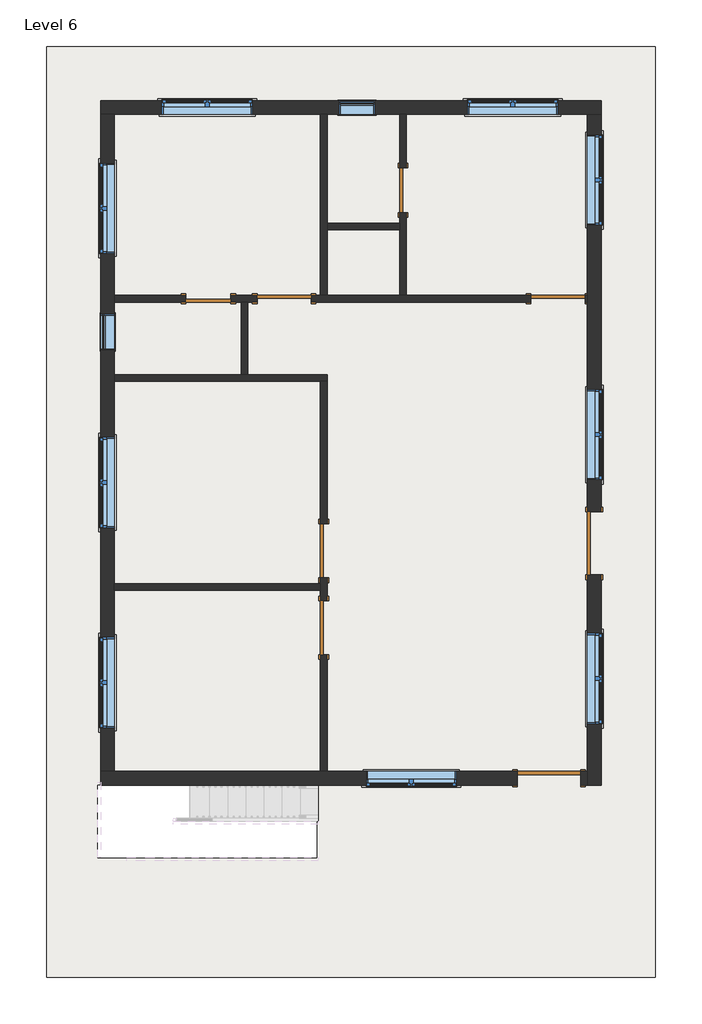
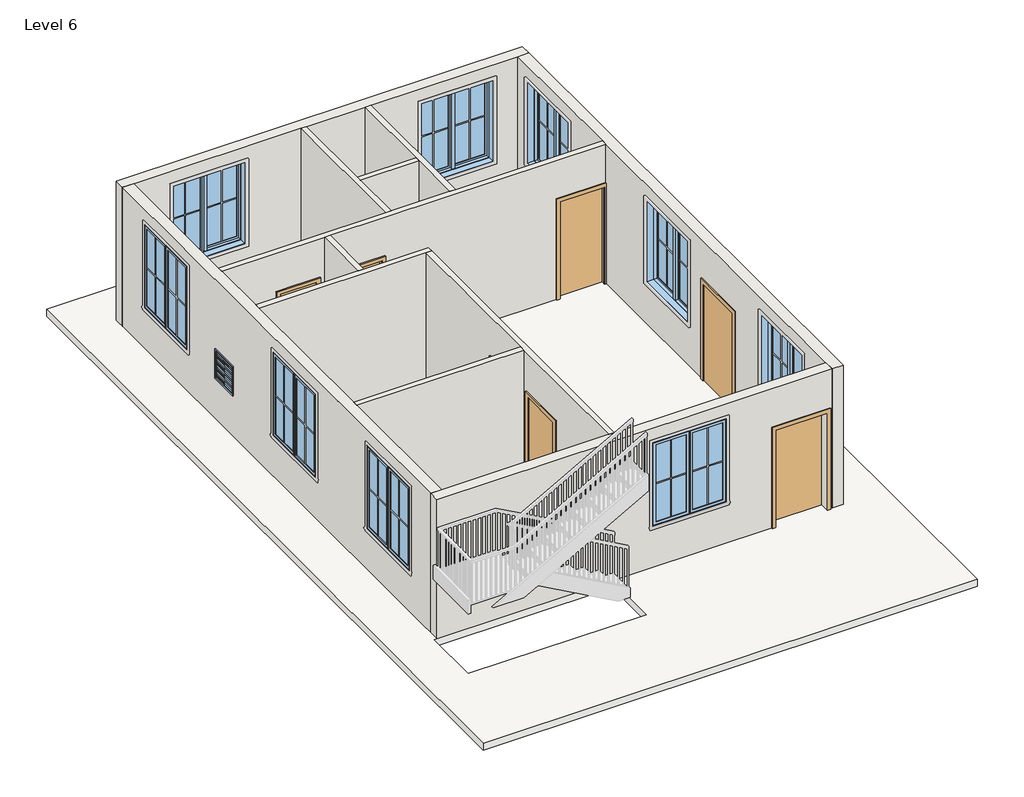
# One storey, part 1 of 3: 12 walls, 11 windows, 8 doors, 1 roof.
"""IFC4 building model written with IfcOpenShell, lengths in millimetres."""

from ifc_helpers import new_model, si_unit, frame, origin, place, context, project, spatial, polyline, outline, extrude, faceted_brep, transform, mapped, element, save
from components import door_78caadf7, single_flush_door_3_e5f9f3c4, single_flush_door_3_305aa2a5, door_9d399b00, door_0848dd25, window_casement_double_win_5_f93960c7, window_f2d8fef0

model = new_model("IFC4")

# Units and contexts
model_context = context("Model", 3, world=origin())
ifc_project = project(units=[si_unit("LENGTHUNIT", "METRE", prefix="MILLI")], contexts=[model_context])

# Site, building, storey
site = spatial("IfcSite", under=ifc_project)
building = spatial("IfcBuilding", under=site)
storey = spatial("IfcBuildingStorey", under=building, Name="Level 6", Elevation=12801.6)

# Doors
placement = place(None, origin())
door_shape = door_78caadf7(model_context)
element("IfcDoor", 1, ObjectType="Single-Flush : DOOR 2'6\"", at=placement, inside=storey, context=model_context, shape_type="MappedRepresentation", body=[
    mapped(door_shape, transform((-377.1698569, 4707.5566963, 12801.6), x_axis=(0.0, -1.0, 0.0), y_axis=(1.0, 0.0, 0.0), z_axis=(0.0, 0.0, 1.0))),
])
element("IfcDoor", 2, ObjectType="Single-Flush : DOOR 2'6\"", at=placement, inside=storey, context=model_context, shape_type="MappedRepresentation", body=[
    mapped(door_shape, transform((-3653.7698569, 2878.7566963, 12801.6), x_axis=(1.0, 0.0, 0.0), y_axis=(0.0, 1.0, 0.0), z_axis=(0.0, 0.0, 1.0))),
])
single_flush_door_3_shape = single_flush_door_3_e5f9f3c4(model_context)
element("IfcDoor", 3, ObjectType="Single-Flush : DOOR 3'", at=placement, inside=storey, context=model_context, shape_type="MappedRepresentation", body=[
    mapped(single_flush_door_3_shape, transform((-2377.4198569, 2878.7566963, 12801.6), x_axis=(1.0, 0.0, 0.0), y_axis=(0.0, 1.0, 0.0), z_axis=(0.0, 0.0, 1.0))),
])
element("IfcDoor", 4, ObjectType="Single-Flush : DOOR 3'", at=placement, inside=storey, context=model_context, shape_type="MappedRepresentation", body=[
    mapped(single_flush_door_3_shape, transform((2232.6801431, 2878.7566963, 12801.6), x_axis=(1.0, 0.0, 0.0), y_axis=(0.0, 1.0, 0.0), z_axis=(0.0, 0.0, 1.0))),
])
element("IfcDoor", 5, ObjectType="Single-Flush : DOOR 3'", at=placement, inside=storey, context=model_context, shape_type="MappedRepresentation", body=[
    mapped(single_flush_door_3_shape, transform((-1710.6698569, -2658.4433037, 12801.6), x_axis=(0.0, 1.0, 0.0), y_axis=(-1.0, 0.0, 0.0), z_axis=(0.0, 0.0, 1.0))),
])
single_flush_door_3_2_shape = single_flush_door_3_305aa2a5(model_context)
element("IfcDoor", 6, ObjectType="Single-Flush : DOOR 3'", at=placement, inside=storey, context=model_context, shape_type="MappedRepresentation", body=[
    mapped(single_flush_door_3_2_shape, transform((-1710.6698569, -1363.0433037, 12801.6), x_axis=(0.0, -1.0, 0.0), y_axis=(1.0, 0.0, 0.0), z_axis=(0.0, 0.0, 1.0))),
])
door_2_shape = door_9d399b00(model_context)
element("IfcDoor", 7, ObjectType="Single-Flush : DOOR 3'6\"", at=placement, inside=storey, context=model_context, shape_type="MappedRepresentation", body=[
    mapped(door_2_shape, transform((2080.2801431, -5192.0933037, 12801.6), x_axis=(1.0, 0.0, 0.0), y_axis=(0.0, 1.0, 0.0), z_axis=(0.0, 0.0, 1.0))),
])
door_3_shape = door_0848dd25(model_context)
element("IfcDoor", 8, ObjectType="Single-Flush : DOOR 3'6\"", at=placement, inside=storey, context=model_context, shape_type="MappedRepresentation", body=[
    mapped(door_3_shape, transform((2842.2801431, -1236.0433037, 12801.6), x_axis=(0.0, -1.0, 0.0), y_axis=(1.0, 0.0, 0.0), z_axis=(0.0, 0.0, 1.0))),
])

# Roof
element("IfcRoof", 9, ObjectType="ROOF 6\"", at=placement, inside=storey, context=model_context, shape_type="SweptSolid", body=[
    extrude(outline(polyline([(-6377.9198569, -8544.8933037), (-6377.9198569, 7126.9066963), (3870.9801431, 7126.9066963), (3870.9801431, -8544.8933037), (-6377.9198569, -8544.8933037)]), holes=[polyline([(-5514.3198569, -5306.3933037), (-5514.3198569, -6525.5933037), (-1831.3198569, -6525.5933037), (-1831.3198569, -5306.3933037), (-5514.3198569, -5306.3933037)])]), frame((0.0, 0.0, 12649.2), z_axis=(0.0, 0.0, 1.0), x_axis=(1.0, 0.0, 0.0)), (0.0, 0.0, 1.0), 152.4),
])

# Walls
element("IfcWall", 10, ObjectType="WALL 4.5\"", at=placement, inside=storey, context=model_context, shape_type="Brep", body=[
    faceted_brep([(2689.8801431, 2821.6066963, 14935.2), (2689.8801431, 2821.6066963, 12801.6), (2727.9801431, 2821.6066963, 12801.6), (2727.9801431, 2821.6066963, 15849.6), (-2987.0198569, 2821.6066963, 15849.6), (-3101.3198569, 2821.6066963, 15849.6), (-5234.9198569, 2821.6066963, 15849.6), (-5234.9198569, 2821.6066963, 12801.6), (-4034.7698569, 2821.6066963, 12801.6), (-4034.7698569, 2821.6066963, 14935.2), (-3272.7698569, 2821.6066963, 14935.2), (-3272.7698569, 2821.6066963, 12801.6), (-3101.3198569, 2821.6066963, 12801.6), (-2987.0198569, 2821.6066963, 12801.6), (-2834.6198569, 2821.6066963, 12801.6), (-2834.6198569, 2821.6066963, 14935.2), (-1920.2198569, 2821.6066963, 14935.2), (-1920.2198569, 2821.6066963, 12801.6), (1775.4801431, 2821.6066963, 12801.6), (1775.4801431, 2821.6066963, 14935.2), (2727.9801431, 2935.9066963, 12801.6), (2689.8801431, 2935.9066963, 12801.6), (2689.8801431, 2935.9066963, 14935.2), (1775.4801431, 2935.9066963, 14935.2), (1775.4801431, 2935.9066963, 12801.6), (-320.0198569, 2935.9066963, 12801.6), (-434.3198569, 2935.9066963, 12801.6), (-1653.5198569, 2935.9066963, 12801.6), (-1767.8198569, 2935.9066963, 12801.6), (-1920.2198569, 2935.9066963, 12801.6), (-1920.2198569, 2935.9066963, 14935.2), (-2834.6198569, 2935.9066963, 14935.2), (-2834.6198569, 2935.9066963, 12801.6), (-3272.7698569, 2935.9066963, 12801.6), (-3272.7698569, 2935.9066963, 14935.2), (-4034.7698569, 2935.9066963, 14935.2), (-4034.7698569, 2935.9066963, 12801.6), (-5234.9198569, 2935.9066963, 12801.6), (-5234.9198569, 2935.9066963, 15849.6), (-1767.8198569, 2935.9066963, 15849.6), (-1653.5198569, 2935.9066963, 15849.6), (-434.3198569, 2935.9066963, 15849.6), (-320.0198569, 2935.9066963, 15849.6), (2727.9801431, 2935.9066963, 15849.6)], [[[0, 1, 2, 3, 4, 5, 6, 7, 8, 9, 10, 11, 12, 13, 14, 15, 16, 17, 18, 19]], [[20, 21, 22, 23, 24, 25, 26, 27, 28, 29, 30, 31, 32, 33, 34, 35, 36, 37, 38, 39, 40, 41, 42, 43]], [[8, 7, 37, 36]], [[14, 13, 12, 11, 33, 32]], [[18, 17, 29, 28, 27, 26, 25, 24]], [[2, 1, 21, 20]], [[3, 2, 20, 43]], [[7, 6, 38, 37]], [[34, 33, 11, 10]], [[35, 34, 10, 9]], [[36, 35, 9, 8]], [[30, 29, 17, 16]], [[31, 30, 16, 15]], [[32, 31, 15, 14]], [[22, 21, 1, 0]], [[23, 22, 0, 19]], [[24, 23, 19, 18]], [[6, 5, 4, 3, 43, 42, 41, 40, 39, 38]]]),
])
element("IfcWall", 11, ObjectType="WALL 4.5\"", at=placement, inside=storey, context=model_context, shape_type="Brep", body=[
    faceted_brep([(-1767.8198569, 5983.9066963, 12801.6), (-1767.8198569, 2935.9066963, 12801.6), (-1767.8198569, 2935.9066963, 15849.6), (-1767.8198569, 5983.9066963, 15849.6), (-1653.5198569, 5983.9066963, 12801.6), (-1653.5198569, 5983.9066963, 15849.6), (-1653.5198569, 4155.1066963, 15849.6), (-1653.5198569, 4040.8066963, 15849.6), (-1653.5198569, 2935.9066963, 15849.6), (-1653.5198569, 2935.9066963, 12801.6), (-1653.5198569, 4040.8066963, 12801.6), (-1653.5198569, 4155.1066963, 12801.6)], [[[0, 1, 2, 3]], [[4, 5, 6, 7, 8, 9, 10, 11]], [[1, 0, 4, 11, 10, 9]], [[0, 3, 5, 4]], [[2, 1, 9, 8]], [[3, 2, 8, 7, 6, 5]]]),
])
element("IfcWall", 12, ObjectType="WALL 4.5\"", at=placement, inside=storey, context=model_context, shape_type="Brep", body=[
    faceted_brep([(-320.0198569, 2935.9066963, 12801.6), (-320.0198569, 4326.5566963, 12801.6), (-320.0198569, 4326.5566963, 14935.2), (-320.0198569, 5088.5566963, 14935.2), (-320.0198569, 5088.5566963, 12801.6), (-320.0198569, 5983.9066963, 12801.6), (-320.0198569, 5983.9066963, 15849.6), (-320.0198569, 2935.9066963, 15849.6), (-434.3198569, 4326.5566963, 14935.2), (-434.3198569, 4326.5566963, 12801.6), (-434.3198569, 4155.1066963, 12801.6), (-434.3198569, 4040.8066963, 12801.6), (-434.3198569, 2935.9066963, 12801.6), (-434.3198569, 2935.9066963, 15849.6), (-434.3198569, 4040.8066963, 15849.6), (-434.3198569, 4155.1066963, 15849.6), (-434.3198569, 5983.9066963, 15849.6), (-434.3198569, 5983.9066963, 12801.6), (-434.3198569, 5088.5566963, 12801.6), (-434.3198569, 5088.5566963, 14935.2)], [[[0, 1, 2, 3, 4, 5, 6, 7]], [[8, 9, 10, 11, 12, 13, 14, 15, 16, 17, 18, 19]], [[18, 17, 5, 4]], [[12, 11, 10, 9, 1, 0]], [[6, 5, 17, 16]], [[0, 7, 13, 12]], [[2, 1, 9, 8]], [[3, 2, 8, 19]], [[4, 3, 19, 18]], [[7, 6, 16, 15, 14, 13]]]),
])
element("IfcWall", 13, ObjectType="WALL 4.5\"", at=placement, inside=storey, context=model_context, shape_type="SweptSolid", body=[
    extrude(outline(polyline([(-434.3198569, 4040.8066963), (-1653.5198569, 4040.8066963), (-1653.5198569, 4155.1066963), (-434.3198569, 4155.1066963), (-434.3198569, 4040.8066963)])), frame((0.0, 0.0, 12801.6), z_axis=(0.0, 0.0, 1.0), x_axis=(1.0, 0.0, 0.0)), (0.0, 0.0, 1.0), 3048.0),
])
element("IfcWall", 14, ObjectType="WALL 4.5\"", at=placement, inside=storey, context=model_context, shape_type="Brep", body=[
    faceted_brep([(-5234.9198569, 1488.1066963, 12801.6), (-1767.8198569, 1488.1066963, 12801.6), (-1653.5198569, 1488.1066963, 12801.6), (-1653.5198569, 1488.1066963, 15849.6), (-1767.8198569, 1488.1066963, 15849.6), (-5234.9198569, 1488.1066963, 15849.6), (-5234.9198569, 1602.4066963, 12801.6), (-5234.9198569, 1602.4066963, 15849.6), (-3101.3198569, 1602.4066963, 15849.6), (-2987.0198569, 1602.4066963, 15849.6), (-1653.5198569, 1602.4066963, 15849.6), (-1653.5198569, 1602.4066963, 12801.6), (-2987.0198569, 1602.4066963, 12801.6), (-3101.3198569, 1602.4066963, 12801.6)], [[[0, 1, 2, 3, 4, 5]], [[6, 7, 8, 9, 10, 11, 12, 13]], [[2, 1, 0, 6, 13, 12, 11]], [[0, 5, 7, 6]], [[3, 2, 11, 10]], [[5, 4, 3, 10, 9, 8, 7]]]),
])
element("IfcWall", 15, ObjectType="WALL 4.5\"", at=placement, inside=storey, context=model_context, shape_type="Brep", body=[
    faceted_brep([(-1767.8198569, -1820.2433037, 12801.6), (-1767.8198569, -1915.4933037, 12801.6), (-1767.8198569, -2029.7933037, 12801.6), (-1767.8198569, -2201.2433037, 12801.6), (-1767.8198569, -2201.2433037, 14935.2), (-1767.8198569, -3115.6433037, 14935.2), (-1767.8198569, -3115.6433037, 12801.6), (-1767.8198569, -5077.7933037, 12801.6), (-1767.8198569, -5077.7933037, 15849.6), (-1767.8198569, -2029.7933037, 15849.6), (-1767.8198569, -1915.4933037, 15849.6), (-1767.8198569, 1488.1066963, 15849.6), (-1767.8198569, 1488.1066963, 12801.6), (-1767.8198569, -905.8433037, 12801.6), (-1767.8198569, -905.8433037, 14935.2), (-1767.8198569, -1820.2433037, 14935.2), (-1653.5198569, -2201.2433037, 14935.2), (-1653.5198569, -2201.2433037, 12801.6), (-1653.5198569, -1820.2433037, 12801.6), (-1653.5198569, -1820.2433037, 14935.2), (-1653.5198569, -905.8433037, 14935.2), (-1653.5198569, -905.8433037, 12801.6), (-1653.5198569, 1488.1066963, 12801.6), (-1653.5198569, 1488.1066963, 15849.6), (-1653.5198569, -5077.7933037, 15849.6), (-1653.5198569, -5077.7933037, 12801.6), (-1653.5198569, -3115.6433037, 12801.6), (-1653.5198569, -3115.6433037, 14935.2)], [[[0, 1, 2, 3, 4, 5, 6, 7, 8, 9, 10, 11, 12, 13, 14, 15]], [[16, 17, 18, 19, 20, 21, 22, 23, 24, 25, 26, 27]], [[13, 12, 22, 21]], [[26, 25, 7, 6]], [[18, 17, 3, 2, 1, 0]], [[12, 11, 23, 22]], [[8, 7, 25, 24]], [[19, 18, 0, 15]], [[20, 19, 15, 14]], [[21, 20, 14, 13]], [[4, 3, 17, 16]], [[5, 4, 16, 27]], [[6, 5, 27, 26]], [[11, 10, 9, 8, 24, 23]]]),
])
element("IfcWall", 16, ObjectType="WALL 4.5\"", at=placement, inside=storey, context=model_context, shape_type="SweptSolid", body=[
    extrude(outline(polyline([(-1767.8198569, -2029.7933037), (-5234.9198569, -2029.7933037), (-5234.9198569, -1915.4933037), (-1767.8198569, -1915.4933037), (-1767.8198569, -2029.7933037)])), frame((0.0, 0.0, 12801.6), z_axis=(0.0, 0.0, 1.0), x_axis=(1.0, 0.0, 0.0)), (0.0, 0.0, 1.0), 3048.0),
])
element("IfcWall", 17, ObjectType="WALL 4.5\"", at=placement, inside=storey, context=model_context, shape_type="SweptSolid", body=[
    extrude(outline(polyline([(-3101.3198569, 1602.4066963), (-3101.3198569, 2821.6066963), (-2987.0198569, 2821.6066963), (-2987.0198569, 1602.4066963), (-3101.3198569, 1602.4066963)])), frame((0.0, 0.0, 12801.6), z_axis=(0.0, 0.0, 1.0), x_axis=(1.0, 0.0, 0.0)), (0.0, 0.0, 1.0), 3048.0),
])
element("IfcWall", 18, ObjectType="WALL 9\"", at=placement, inside=storey, context=model_context, shape_type="Brep", body=[
    faceted_brep([(-5463.5198569, 5983.9066963, 12801.6), (-5234.9198569, 5983.9066963, 12801.6), (-1767.8198569, 5983.9066963, 12801.6), (-1653.5198569, 5983.9066963, 12801.6), (-434.3198569, 5983.9066963, 12801.6), (-320.0198569, 5983.9066963, 12801.6), (2727.9801431, 5983.9066963, 12801.6), (2956.5801431, 5983.9066963, 12801.6), (2956.5801431, 5983.9066963, 15849.6), (2727.9801431, 5983.9066963, 15849.6), (-320.0198569, 5983.9066963, 15849.6), (-434.3198569, 5983.9066963, 15849.6), (-1653.5198569, 5983.9066963, 15849.6), (-1767.8198569, 5983.9066963, 15849.6), (-5234.9198569, 5983.9066963, 15849.6), (-5463.5198569, 5983.9066963, 15849.6), (2232.6801431, 5983.9066963, 15544.8), (2232.6801431, 5983.9066963, 13716.0), (708.6801431, 5983.9066963, 13716.0), (708.6801431, 5983.9066963, 15544.8), (-2910.8198569, 5983.9066963, 15544.8), (-2910.8198569, 5983.9066963, 13716.0), (-4434.8198569, 5983.9066963, 13716.0), (-4434.8198569, 5983.9066963, 15544.8), (-1456.6698569, 5983.9066963, 14325.6), (-847.0698569, 5983.9066963, 14325.6), (-847.0698569, 5983.9066963, 13716.0), (-1456.6698569, 5983.9066963, 13716.0), (-5463.5198569, 6212.5066963, 12801.6), (-5463.5198569, 6212.5066963, 15849.6), (2956.5801431, 6212.5066963, 15849.6), (2956.5801431, 6212.5066963, 12801.6), (2232.6801431, 6212.5066963, 15544.8), (708.6801431, 6212.5066963, 15544.8), (708.6801431, 6212.5066963, 13716.0), (2232.6801431, 6212.5066963, 13716.0), (-2910.8198569, 6212.5066963, 15544.8), (-4434.8198569, 6212.5066963, 15544.8), (-4434.8198569, 6212.5066963, 13716.0), (-2910.8198569, 6212.5066963, 13716.0), (-1456.6698569, 6212.5066963, 14325.6), (-1456.6698569, 6212.5066963, 13716.0), (-847.0698569, 6212.5066963, 13716.0), (-847.0698569, 6212.5066963, 14325.6)], [[[0, 1, 2, 3, 4, 5, 6, 7, 8, 9, 10, 11, 12, 13, 14, 15], [16, 17, 18, 19], [20, 21, 22, 23], [24, 25, 26, 27]], [[28, 29, 30, 31], [32, 33, 34, 35], [36, 37, 38, 39], [40, 41, 42, 43]], [[7, 6, 5, 4, 3, 2, 1, 0, 28, 31]], [[8, 7, 31, 30]], [[0, 15, 29, 28]], [[17, 16, 32, 35]], [[18, 17, 35, 34]], [[19, 18, 34, 33]], [[16, 19, 33, 32]], [[21, 20, 36, 39]], [[22, 21, 39, 38]], [[23, 22, 38, 37]], [[20, 23, 37, 36]], [[41, 40, 24, 27]], [[42, 41, 27, 26]], [[43, 42, 26, 25]], [[40, 43, 25, 24]], [[15, 14, 13, 12, 11, 10, 9, 8, 30, 29]]]),
])
element("IfcWall", 19, ObjectType="WALL 9\"", at=placement, inside=storey, context=model_context, shape_type="Brep", body=[
    faceted_brep([(2727.9801431, -1769.4433037, 14935.2), (2727.9801431, -1769.4433037, 12801.6), (2727.9801431, -5077.7933037, 12801.6), (2727.9801431, -5306.3933037, 12801.6), (2727.9801431, -5306.3933037, 15849.6), (2727.9801431, -5077.7933037, 15849.6), (2727.9801431, 2821.6066963, 15849.6), (2727.9801431, 2935.9066963, 15849.6), (2727.9801431, 5983.9066963, 15849.6), (2727.9801431, 5983.9066963, 12801.6), (2727.9801431, 2935.9066963, 12801.6), (2727.9801431, 2821.6066963, 12801.6), (2727.9801431, -702.6433037, 12801.6), (2727.9801431, -702.6433037, 14935.2), (2727.9801431, 4117.0066963, 15544.8), (2727.9801431, 4117.0066963, 13716.0), (2727.9801431, 5641.0066963, 13716.0), (2727.9801431, 5641.0066963, 15544.8), (2727.9801431, -169.2433037, 15544.8), (2727.9801431, -169.2433037, 13716.0), (2727.9801431, 1354.7566963, 13716.0), (2727.9801431, 1354.7566963, 15544.8), (2727.9801431, -4277.6933037, 15544.8), (2727.9801431, -4277.6933037, 13716.0), (2727.9801431, -2753.6933037, 13716.0), (2727.9801431, -2753.6933037, 15544.8), (2956.5801431, -5306.3933037, 12801.6), (2956.5801431, -1769.4433037, 12801.6), (2956.5801431, -1769.4433037, 14935.2), (2956.5801431, -702.6433037, 14935.2), (2956.5801431, -702.6433037, 12801.6), (2956.5801431, 5983.9066963, 12801.6), (2956.5801431, 5983.9066963, 15849.6), (2956.5801431, -5306.3933037, 15849.6), (2956.5801431, 4117.0066963, 15544.8), (2956.5801431, 5641.0066963, 15544.8), (2956.5801431, 5641.0066963, 13716.0), (2956.5801431, 4117.0066963, 13716.0), (2956.5801431, -169.2433037, 15544.8), (2956.5801431, 1354.7566963, 15544.8), (2956.5801431, 1354.7566963, 13716.0), (2956.5801431, -169.2433037, 13716.0), (2956.5801431, -4277.6933037, 15544.8), (2956.5801431, -2753.6933037, 15544.8), (2956.5801431, -2753.6933037, 13716.0), (2956.5801431, -4277.6933037, 13716.0)], [[[0, 1, 2, 3, 4, 5, 6, 7, 8, 9, 10, 11, 12, 13], [14, 15, 16, 17], [18, 19, 20, 21], [22, 23, 24, 25]], [[26, 27, 28, 29, 30, 31, 32, 33], [34, 35, 36, 37], [38, 39, 40, 41], [42, 43, 44, 45]], [[3, 2, 1, 27, 26]], [[12, 11, 10, 9, 31, 30]], [[9, 8, 32, 31]], [[4, 3, 26, 33]], [[15, 14, 34, 37]], [[16, 15, 37, 36]], [[17, 16, 36, 35]], [[14, 17, 35, 34]], [[19, 18, 38, 41]], [[20, 19, 41, 40]], [[21, 20, 40, 39]], [[18, 21, 39, 38]], [[23, 22, 42, 45]], [[24, 23, 45, 44]], [[25, 24, 44, 43]], [[22, 25, 43, 42]], [[28, 27, 1, 0]], [[29, 28, 0, 13]], [[30, 29, 13, 12]], [[8, 7, 6, 5, 4, 33, 32]]]),
])
element("IfcWall", 20, ObjectType="WALL 9\"", at=placement, inside=storey, context=model_context, shape_type="Brep", body=[
    faceted_brep([(2727.9801431, -5077.7933037, 12801.6), (2613.6801431, -5077.7933037, 12801.6), (2613.6801431, -5077.7933037, 14935.2), (1546.8801431, -5077.7933037, 14935.2), (1546.8801431, -5077.7933037, 12801.6), (-1653.5198569, -5077.7933037, 12801.6), (-1767.8198569, -5077.7933037, 12801.6), (-5234.9198569, -5077.7933037, 12801.6), (-5463.5198569, -5077.7933037, 12801.6), (-5463.5198569, -5077.7933037, 15849.6), (-5234.9198569, -5077.7933037, 15849.6), (-1767.8198569, -5077.7933037, 15849.6), (-1653.5198569, -5077.7933037, 15849.6), (2727.9801431, -5077.7933037, 15849.6), (-999.4698569, -5077.7933037, 15544.8), (-999.4698569, -5077.7933037, 13716.0), (524.5301431, -5077.7933037, 13716.0), (524.5301431, -5077.7933037, 15544.8), (2613.6801431, -5306.3933037, 14935.2), (2613.6801431, -5306.3933037, 12801.6), (2727.9801431, -5306.3933037, 12801.6), (2727.9801431, -5306.3933037, 15849.6), (-1831.3198569, -5306.3933037, 15849.6), (-5463.5198569, -5306.3933037, 15849.6), (-5463.5198569, -5306.3933037, 12801.6), (1546.8801431, -5306.3933037, 12801.6), (1546.8801431, -5306.3933037, 14935.2), (-999.4698569, -5306.3933037, 15544.8), (524.5301431, -5306.3933037, 15544.8), (524.5301431, -5306.3933037, 13716.0), (-999.4698569, -5306.3933037, 13716.0)], [[[0, 1, 2, 3, 4, 5, 6, 7, 8, 9, 10, 11, 12, 13], [14, 15, 16, 17]], [[18, 19, 20, 21, 22, 23, 24, 25, 26], [27, 28, 29, 30]], [[25, 24, 8, 7, 6, 5, 4]], [[20, 19, 1, 0]], [[0, 13, 21, 20]], [[9, 8, 24, 23]], [[15, 14, 27, 30]], [[16, 15, 30, 29]], [[17, 16, 29, 28]], [[14, 17, 28, 27]], [[2, 1, 19, 18]], [[3, 2, 18, 26]], [[4, 3, 26, 25]], [[13, 12, 11, 10, 9, 23, 22, 21]]]),
])
element("IfcWall", 21, ObjectType="WALL 9\"", at=placement, inside=storey, context=model_context, shape_type="Brep", body=[
    faceted_brep([(-5234.9198569, -5077.7933037, 12801.6), (-5234.9198569, -2029.7933037, 12801.6), (-5234.9198569, -1915.4933037, 12801.6), (-5234.9198569, 1488.1066963, 12801.6), (-5234.9198569, 1602.4066963, 12801.6), (-5234.9198569, 2821.6066963, 12801.6), (-5234.9198569, 2935.9066963, 12801.6), (-5234.9198569, 5983.9066963, 12801.6), (-5234.9198569, 5983.9066963, 15849.6), (-5234.9198569, 2935.9066963, 15849.6), (-5234.9198569, 2821.6066963, 15849.6), (-5234.9198569, 1602.4066963, 15849.6), (-5234.9198569, 1488.1066963, 15849.6), (-5234.9198569, -1915.4933037, 15849.6), (-5234.9198569, -2029.7933037, 15849.6), (-5234.9198569, -5077.7933037, 15849.6), (-5234.9198569, -2820.3683037, 15544.8), (-5234.9198569, -2820.3683037, 13716.0), (-5234.9198569, -4344.3683037, 13716.0), (-5234.9198569, -4344.3683037, 15544.8), (-5234.9198569, 548.3066963, 15544.8), (-5234.9198569, 548.3066963, 13716.0), (-5234.9198569, -975.6933037, 13716.0), (-5234.9198569, -975.6933037, 15544.8), (-5234.9198569, 5164.7566963, 15544.8), (-5234.9198569, 5164.7566963, 13716.0), (-5234.9198569, 3640.7566963, 13716.0), (-5234.9198569, 3640.7566963, 15544.8), (-5234.9198569, 2015.1566963, 14325.6), (-5234.9198569, 2624.7566963, 14325.6), (-5234.9198569, 2624.7566963, 13716.0), (-5234.9198569, 2015.1566963, 13716.0), (-5463.5198569, -5077.7933037, 12801.6), (-5463.5198569, -5077.7933037, 15849.6), (-5463.5198569, 5983.9066963, 15849.6), (-5463.5198569, 5983.9066963, 12801.6), (-5463.5198569, -2820.3683037, 15544.8), (-5463.5198569, -4344.3683037, 15544.8), (-5463.5198569, -4344.3683037, 13716.0), (-5463.5198569, -2820.3683037, 13716.0), (-5463.5198569, 548.3066963, 15544.8), (-5463.5198569, -975.6933037, 15544.8), (-5463.5198569, -975.6933037, 13716.0), (-5463.5198569, 548.3066963, 13716.0), (-5463.5198569, 5164.7566963, 15544.8), (-5463.5198569, 3640.7566963, 15544.8), (-5463.5198569, 3640.7566963, 13716.0), (-5463.5198569, 5164.7566963, 13716.0), (-5463.5198569, 2015.1566963, 14325.6), (-5463.5198569, 2015.1566963, 13716.0), (-5463.5198569, 2624.7566963, 13716.0), (-5463.5198569, 2624.7566963, 14325.6)], [[[0, 1, 2, 3, 4, 5, 6, 7, 8, 9, 10, 11, 12, 13, 14, 15], [16, 17, 18, 19], [20, 21, 22, 23], [24, 25, 26, 27], [28, 29, 30, 31]], [[32, 33, 34, 35], [36, 37, 38, 39], [40, 41, 42, 43], [44, 45, 46, 47], [48, 49, 50, 51]], [[7, 6, 5, 4, 3, 2, 1, 0, 32, 35]], [[8, 7, 35, 34]], [[0, 15, 33, 32]], [[17, 16, 36, 39]], [[18, 17, 39, 38]], [[19, 18, 38, 37]], [[16, 19, 37, 36]], [[21, 20, 40, 43]], [[22, 21, 43, 42]], [[23, 22, 42, 41]], [[20, 23, 41, 40]], [[25, 24, 44, 47]], [[26, 25, 47, 46]], [[27, 26, 46, 45]], [[24, 27, 45, 44]], [[49, 48, 28, 31]], [[50, 49, 31, 30]], [[51, 50, 30, 29]], [[48, 51, 29, 28]], [[15, 14, 13, 12, 11, 10, 9, 8, 34, 33]]]),
])

# Windows
window_casement_double_win_5_shape = window_casement_double_win_5_f93960c7(model_context)
element("IfcWindow", 22, ObjectType="Window-Casement-Double : WIN 5'", at=placement, inside=storey, context=model_context, shape_type="MappedRepresentation", body=[
    mapped(window_casement_double_win_5_shape, transform((-5349.2198569, -3582.3683037, 12801.6), x_axis=(0.0, 1.0, 0.0), y_axis=(-1.0, 0.0, 0.0), z_axis=(0.0, 0.0, 1.0))),
])
element("IfcWindow", 23, ObjectType="Window-Casement-Double : WIN 5'", at=placement, inside=storey, context=model_context, shape_type="MappedRepresentation", body=[
    mapped(window_casement_double_win_5_shape, transform((-5349.2198569, -213.6933037, 12801.6), x_axis=(0.0, 1.0, 0.0), y_axis=(-1.0, 0.0, 0.0), z_axis=(0.0, 0.0, 1.0))),
])
element("IfcWindow", 24, ObjectType="Window-Casement-Double : WIN 5'", at=placement, inside=storey, context=model_context, shape_type="MappedRepresentation", body=[
    mapped(window_casement_double_win_5_shape, transform((-5349.2198569, 4402.7566963, 12801.6), x_axis=(0.0, 1.0, 0.0), y_axis=(-1.0, 0.0, 0.0), z_axis=(0.0, 0.0, 1.0))),
])
element("IfcWindow", 25, ObjectType="Window-Casement-Double : WIN 5'", at=placement, inside=storey, context=model_context, shape_type="MappedRepresentation", body=[
    mapped(window_casement_double_win_5_shape, transform((2842.2801431, 4879.0066963, 12801.6), x_axis=(0.0, -1.0, 0.0), y_axis=(1.0, 0.0, 0.0), z_axis=(0.0, 0.0, 1.0))),
])
element("IfcWindow", 26, ObjectType="Window-Casement-Double : WIN 5'", at=placement, inside=storey, context=model_context, shape_type="MappedRepresentation", body=[
    mapped(window_casement_double_win_5_shape, transform((2842.2801431, 592.7566963, 12801.6), x_axis=(0.0, -1.0, 0.0), y_axis=(1.0, 0.0, 0.0), z_axis=(0.0, 0.0, 1.0))),
])
element("IfcWindow", 27, ObjectType="Window-Casement-Double : WIN 5'", at=placement, inside=storey, context=model_context, shape_type="MappedRepresentation", body=[
    mapped(window_casement_double_win_5_shape, transform((2842.2801431, -3515.6933037, 12801.6), x_axis=(0.0, -1.0, 0.0), y_axis=(1.0, 0.0, 0.0), z_axis=(0.0, 0.0, 1.0))),
])
element("IfcWindow", 28, ObjectType="Window-Casement-Double : WIN 5'", at=placement, inside=storey, context=model_context, shape_type="MappedRepresentation", body=[
    mapped(window_casement_double_win_5_shape, transform((-237.4698569, -5192.0933037, 12801.6), x_axis=(-1.0, 0.0, 0.0), y_axis=(0.0, -1.0, 0.0), z_axis=(0.0, 0.0, 1.0))),
])
element("IfcWindow", 29, ObjectType="Window-Casement-Double : WIN 5'", at=placement, inside=storey, context=model_context, shape_type="MappedRepresentation", body=[
    mapped(window_casement_double_win_5_shape, transform((1470.6801431, 6098.2066963, 12801.6), x_axis=(1.0, 0.0, 0.0), y_axis=(0.0, 1.0, 0.0), z_axis=(0.0, 0.0, 1.0))),
])
element("IfcWindow", 30, ObjectType="Window-Casement-Double : WIN 5'", at=placement, inside=storey, context=model_context, shape_type="MappedRepresentation", body=[
    mapped(window_casement_double_win_5_shape, transform((-3672.8198569, 6098.2066963, 12801.6), x_axis=(1.0, 0.0, 0.0), y_axis=(0.0, 1.0, 0.0), z_axis=(0.0, 0.0, 1.0))),
])
window_shape = window_f2d8fef0(model_context)
element("IfcWindow", 31, ObjectType="Window-Louvers : 24\" x 24\"", at=placement, inside=storey, context=model_context, shape_type="MappedRepresentation", body=[
    mapped(window_shape, transform((-1151.8698569, 6104.5566963, 12801.6), x_axis=(1.0, 0.0, 0.0), y_axis=(0.0, 1.0, 0.0), z_axis=(0.0, 0.0, 1.0))),
])
element("IfcWindow", 32, ObjectType="Window-Louvers : 24\" x 24\"", at=placement, inside=storey, context=model_context, shape_type="MappedRepresentation", body=[
    mapped(window_shape, transform((-5355.5698569, 2319.9566963, 12801.6), x_axis=(0.0, 1.0, 0.0), y_axis=(-1.0, 0.0, 0.0), z_axis=(0.0, 0.0, 1.0))),
])

save(model, "model.ifc")

# Revit data of these elements
# Type "Single-Flush : DOOR 2'6\""
#   Type Mark = "10"
#   Construction Type Id = "MDOOR"
#   Assembly Code = "C1020"
#   Analytic Construction = "Metal"
#   Thickness = 0' - 2"
#   Heat Transfer Coefficient (U) = 0.651978 BTU/(h·ft²·°F)
#   Height = 7' - 0"
#   Trim Projection Ext = 0' - 1"
#   Trim Projection Int = 0' - 1"
#   Trim Width = 0' - 3"
#   Width = 2' - 6"
#   Define Thermal Properties by = 1
#   Door Material = Door - Panel
#   Frame Material = Door - Frame
#   Visual Light Transmittance = 0
#   Solar Heat Gain Coefficient = 0
#   Function = (empty or 0)
#   Wall Closure = (empty or 0)
# Type "Single-Flush : DOOR 3'"
#   Type Mark = "8"
#   Construction Type Id = "MDOOR"
#   Assembly Code = "C1020"
#   Analytic Construction = "Metal"
#   Thickness = 0' - 2"
#   Heat Transfer Coefficient (U) = 0.651978 BTU/(h·ft²·°F)
#   Height = 7' - 0"
#   Trim Projection Ext = 0' - 1"
#   Trim Projection Int = 0' - 1"
#   Trim Width = 0' - 3"
#   Width = 3' - 0"
#   Define Thermal Properties by = 1
#   Door Material = Door - Panel
#   Frame Material = Door - Frame
#   Visual Light Transmittance = 0
#   Solar Heat Gain Coefficient = 0
#   Function = (empty or 0)
#   Wall Closure = (empty or 0)
# Type "Single-Flush : DOOR 3'6\""
#   Type Mark = "9"
#   Construction Type Id = "MDOOR"
#   Assembly Code = "C1020"
#   Analytic Construction = "Metal"
#   Thickness = 0' - 2"
#   Heat Transfer Coefficient (U) = 0.651978 BTU/(h·ft²·°F)
#   Height = 7' - 0"
#   Trim Projection Ext = 0' - 1"
#   Trim Projection Int = 0' - 1"
#   Trim Width = 0' - 3"
#   Width = 3' - 6"
#   Define Thermal Properties by = 1
#   Door Material = Door - Panel
#   Frame Material = Door - Frame
#   Visual Light Transmittance = 0
#   Solar Heat Gain Coefficient = 0
#   Function = (empty or 0)
#   Wall Closure = (empty or 0)
# Type "ROOF 6\""
#   Assembly Code = "B1020"
#   Layers, outside or top first: 0' - 6" no material (function 1)
# Type "WALL 4.5\""
#   Assembly Code = "B2010"
#   Layers, outside or top first: 0' - 4 1/2" no material (function 1)
# Type "WALL 9\""
#   Assembly Code = "B2010"
#   Layers, outside or top first: 0' - 9" no material (function 1)
# Type "Window-Casement-Double : WIN 5'"
#   Type Mark = "20"
#   Fire Rating = "0.5h"
#   Assembly Code = "B2020100"
#   Analytic Construction = "Double glazing - domestic"
#   Frame Extension [instance default] = 0' - 0 1/4"
#   Window Inset [instance default] = 0' - 0"
#   Wall Thickness [instance default] = 0' - 6"
#   Interior Wall Closure [instance default] = 0' - 2 1/4"
#   Half Width = 2' - 6"
#   Visual Light Transmittance = 0.81
#   Thermal Resistance (R) = 1.8146 (h·ft²·°F)/BTU
#   Solar Heat Gain Coefficient = 0.76
#   Rough Width = 5' - 0 1/2"
#   Rough Height = 6' - 0 1/2"
#   Height = 6' - 0"
#   Heat Transfer Coefficient (U) = 0.5511 BTU/(h·ft²·°F)
#   Exterior Wall Closure [instance default] = 0' - 1 1/4"
#   Extension Jamb [instance default] = 0' - 2 1/4"
#   Default Sill Height = 3' - 0"
#   Width = 5' - 0"
#   Muntin Visibility = yes
#   Interior Trim Visibility [instance default] = yes
#   Exterior Trim Visibility [instance default] = yes
#   Extension Jamb Visibility [instance default] = yes
#   Interior Trim Material = Wood - Stained
#   Muntin Pattern = Muntin Pattern_2x2 : Muntin Pattern_2x2
#   Interior Trim = Trim-Window-Interior-Flat : Picture Frame
#   Interior Frame Material = Wood - Stained
#   Glass Panel Material = Glass
#   Exterior Trim Material = Clad - White
#   Exterior Trim = Trim-Window-Exterior-Flat : with Sill
#   Exterior Frame Material = Clad - White
#   Wall Closure = (empty or 0)
# Type "Window-Louvers : 24\" x 24\""
#   Type Mark = "21"
#   Construction Type Id = "GSP4R"
#   Assembly Code = "B20"
#   Analytic Construction = "1/8 in Pilkington single glazing"
#   Visual Light Transmittance = 0.9
#   Thermal Resistance (R) = 1.53941 (h·ft²·°F)/BTU
#   Solar Heat Gain Coefficient = 0.78
#   Max Height = 1' - 11.74264"
#   Height = 2' - 0"
#   Heat Transfer Coefficient (U) = 0.6496 BTU/(h·ft²·°F)
#   Blade Width [instance default] = 1' - 10 1/2"
#   Blade Vertical Thickness = 0' - 0.35355"
#   Blade Thickness = 0' - 0 1/4"
#   Blade Spacing = 0' - 1 1/2"
#   Blade Height = 0' - 1.85355"
#   Blade Depth = 0' - 3"
#   Blade Angle = 45.00°
#   Default Sill Height = 3' - 0"
#   Trim Projection_Exterior = 0' - 0 1/2"
#   Trim Projection_Interior = 0' - 0 1/2"
#   Trim Width_Exterior = 0' - 1 1/2"
#   Trim Width_Interior = 0' - 1 1/2"
#   Width = 2' - 0"
#   Max Blade Count = 12
#   Define Thermal Properties by = 1
#   Blade Count = 12
#   Frame Material = Birch
#   Louver Material = Birch
#   Trim Exterior Material = Birch
#   Trim Interior Material = Birch
#   Wall Closure = (empty or 0)
# Elements 1, 2 (IfcDoor, "Single-Flush : DOOR 2'6\"")
#   Phase Created = New Construction
#   Materials on its faces: "Door - Frame", "Door - Panel"
# Elements 3, 4, 5, 6 (IfcDoor, "Single-Flush : DOOR 3'")
#   Phase Created = New Construction
#   Materials on its faces: "Door - Frame", "Door - Panel"
# Elements 7, 8 (IfcDoor, "Single-Flush : DOOR 3'6\"")
#   Phase Created = New Construction
#   Materials on its faces: "Door - Frame", "Door - Panel"
# Element 9 (IfcRoof, "ROOF 6\"")
#   built-in parameter 1001705 = 42 (stored number, unit not read)
#   built-in parameter 1001701 = -0.5 (stored number, unit not read)
#   built-in parameter 1001710 = 33615
#   Phase Created = New Construction
#   Materials on its faces: "Default Roof", "Parking Stripe", "Wood - Stained"
# Elements 10, 11, 12, 13, 14, 15, 16, 17 (IfcWall, "WALL 4.5\"")
#   Top Offset = 0' - 0"
#   Base Offset = 0' - 0"
#   Unconnected Height = 10' - 0"
#   wall height = 10' - 0"
#   Phase Created = New Construction
#   Base Constraint = Level 6
#   Materials on its faces: "Default Wall"
# Elements 18, 19, 20, 21 (IfcWall, "WALL 9\"")
#   Top Offset = 0' - 0"
#   Base Offset = 0' - 0"
#   Unconnected Height = 10' - 0"
#   wall height = 10' - 0"
#   Phase Created = New Construction
#   Base Constraint = Level 6
#   Materials on its faces: "Default Wall", "Cherry"
# Element 22 (IfcWindow, "Window-Casement-Double : WIN 5'")
#   Mark = "45"
#   Window Inset = 0' - 0"
#   Interior Wall Closure = 0' - 2 1/4"
#   Frame Extension = 0' - 0 1/4"
#   Exterior Wall Closure = 0' - 1 1/4"
#   Interior Trim Visibility = yes
#   Exterior Trim Visibility = yes
#   Phase Created = New Construction
#   Materials on its faces: "Wood - Stained", "Glass", "Clad - White"
# Element 23 (IfcWindow, "Window-Casement-Double : WIN 5'")
#   Mark = "46"
#   Window Inset = 0' - 0"
#   Interior Wall Closure = 0' - 2 1/4"
#   Frame Extension = 0' - 0 1/4"
#   Exterior Wall Closure = 0' - 1 1/4"
#   Interior Trim Visibility = yes
#   Exterior Trim Visibility = yes
#   Phase Created = New Construction
#   Materials on its faces: "Wood - Stained", "Glass", "Clad - White"
# Element 24 (IfcWindow, "Window-Casement-Double : WIN 5'")
#   Mark = "47"
#   Window Inset = 0' - 0"
#   Interior Wall Closure = 0' - 2 1/4"
#   Frame Extension = 0' - 0 1/4"
#   Exterior Wall Closure = 0' - 1 1/4"
#   Interior Trim Visibility = yes
#   Exterior Trim Visibility = yes
#   Phase Created = New Construction
#   Materials on its faces: "Wood - Stained", "Glass", "Clad - White"
# Element 25 (IfcWindow, "Window-Casement-Double : WIN 5'")
#   Mark = "48"
#   Window Inset = 0' - 0"
#   Interior Wall Closure = 0' - 2 1/4"
#   Frame Extension = 0' - 0 1/4"
#   Exterior Wall Closure = 0' - 1 1/4"
#   Interior Trim Visibility = yes
#   Exterior Trim Visibility = yes
#   Phase Created = New Construction
#   Materials on its faces: "Wood - Stained", "Glass", "Clad - White"
# Element 26 (IfcWindow, "Window-Casement-Double : WIN 5'")
#   Mark = "49"
#   Window Inset = 0' - 0"
#   Interior Wall Closure = 0' - 2 1/4"
#   Frame Extension = 0' - 0 1/4"
#   Exterior Wall Closure = 0' - 1 1/4"
#   Interior Trim Visibility = yes
#   Exterior Trim Visibility = yes
#   Phase Created = New Construction
#   Materials on its faces: "Wood - Stained", "Glass", "Clad - White"
# Element 27 (IfcWindow, "Window-Casement-Double : WIN 5'")
#   Mark = "50"
#   Window Inset = 0' - 0"
#   Interior Wall Closure = 0' - 2 1/4"
#   Frame Extension = 0' - 0 1/4"
#   Exterior Wall Closure = 0' - 1 1/4"
#   Interior Trim Visibility = yes
#   Exterior Trim Visibility = yes
#   Phase Created = New Construction
#   Materials on its faces: "Wood - Stained", "Glass", "Clad - White"
# Element 28 (IfcWindow, "Window-Casement-Double : WIN 5'")
#   Mark = "51"
#   Window Inset = 0' - 0"
#   Interior Wall Closure = 0' - 2 1/4"
#   Frame Extension = 0' - 0 1/4"
#   Exterior Wall Closure = 0' - 1 1/4"
#   Interior Trim Visibility = yes
#   Exterior Trim Visibility = yes
#   Phase Created = New Construction
#   Materials on its faces: "Wood - Stained", "Glass", "Clad - White"
# Element 29 (IfcWindow, "Window-Casement-Double : WIN 5'")
#   Mark = "52"
#   Window Inset = 0' - 0"
#   Interior Wall Closure = 0' - 2 1/4"
#   Frame Extension = 0' - 0 1/4"
#   Exterior Wall Closure = 0' - 1 1/4"
#   Interior Trim Visibility = yes
#   Exterior Trim Visibility = yes
#   Phase Created = New Construction
#   Materials on its faces: "Wood - Stained", "Glass", "Clad - White"
# Element 30 (IfcWindow, "Window-Casement-Double : WIN 5'")
#   Mark = "53"
#   Window Inset = 0' - 0"
#   Interior Wall Closure = 0' - 2 1/4"
#   Frame Extension = 0' - 0 1/4"
#   Exterior Wall Closure = 0' - 1 1/4"
#   Interior Trim Visibility = yes
#   Exterior Trim Visibility = yes
#   Phase Created = New Construction
#   Materials on its faces: "Wood - Stained", "Glass", "Clad - White"
# Element 31 (IfcWindow, "Window-Louvers : 24\" x 24\"")
#   Mark = "54"
#   Blade Width = 1' - 10 1/2"
#   Phase Created = New Construction
#   Materials on its faces: "Birch"
# Element 32 (IfcWindow, "Window-Louvers : 24\" x 24\"")
#   Mark = "55"
#   Blade Width = 1' - 10 1/2"
#   Phase Created = New Construction
#   Materials on its faces: "Birch"
# Materials
#   "Door - Panel": class "Wood", colour RGB 210 159 95, transparency 0, Cost = 0
#   "Door - Frame": colour RGB 118 70 51, transparency 0, Cost = 0
#   "Wood - Stained": class "Wood", colour RGB 224 178 126, transparency 0, Cost = 0
#   "Glass": class "Glass", colour RGB 0 128 192, transparency 0.75, Description = "Soda Lime Glass", Cost = 0
#   "Clad - White": class "Wood", colour RGB 242 242 238, transparency 0, Cost = 0
#   "Birch": class "Wood", colour RGB 224 178 126, transparency 0, Description = "Betula Alleghaniensis", Cost = 0
#   "Default Roof": colour RGB 88 101 114, transparency 0, Cost = 0
#   "Parking Stripe": class "Paint", colour RGB 250 250 91, transparency 0, Cost = 0
#   "Default Wall": colour RGB 128 128 128, transparency 0, Cost = 0
#   "Cherry": class "Wood", colour RGB 226 177 128, transparency 0, Description = "Prunus Serotina", Cost = 0
